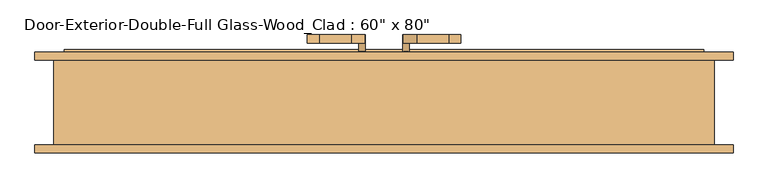
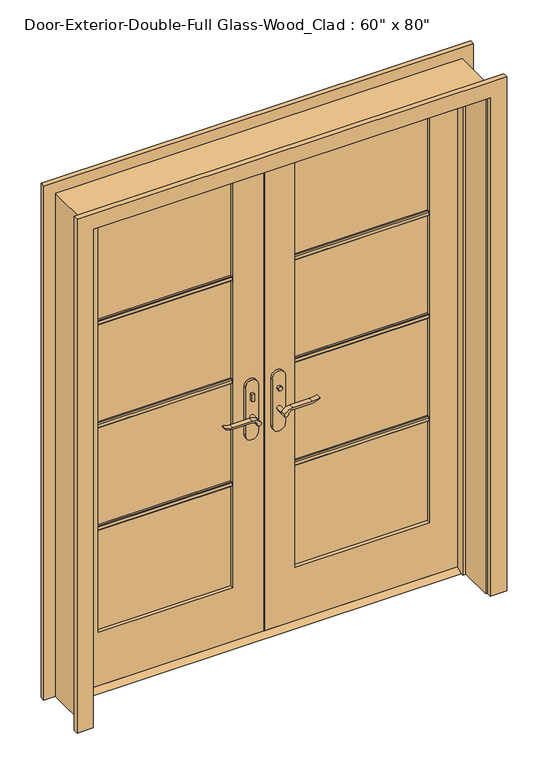
"""IFC4 building model written with IfcOpenShell, lengths in millimetres: door geometry."""

from ifc_helpers import new_model, si_unit, point, frame, frame_2d, origin, place, context, project, spatial, polyline, circle_curve, trimmed, segment, composite_curve, outline, extrude, faceted_brep, source, transform, mapped, element, save


def door_b03bd389(model_context):
    return source(origin(), model_context, "Body", "SolidModel", [
        extrude(outline(polyline([(63.5, 12.7), (98.425, 12.7), (123.825, 0.0), (38.1, 0.0), (63.5, 12.7)])), frame((-762.0, 0.0, 0.0), z_axis=(1.0, 0.0, 0.0), x_axis=(0.0, 1.0, 0.0)), (0.0, 0.0, 1.0), 1524.0),
        extrude(outline(polyline([(-47.4019111, 43.5), (-57.4019111, 43.5), (-57.4019111, 53.5), (-47.4019111, 53.5), (-47.4019111, 43.5)])), frame((0.0, 0.0, 981.9), z_axis=(0.0, 0.0, 1.0), x_axis=(1.0, 0.0, 0.0)), (0.0, 0.0, 1.0), 30.0),
        extrude(outline(composite_curve([segment(trimmed(circle_curve(frame_2d((996.9, -52.4019111)), 8.0), [point((996.9, -60.4019111))], [point((996.9, -44.4019111))], False, "CARTESIAN"), True, "CONTINUOUS"), segment(trimmed(circle_curve(frame_2d((996.9, -52.4019111)), 8.0), [point((996.9, -44.4019111))], [point((996.9, -60.4019111))], False, "CARTESIAN"), True, "CONTINUOUS")], self_intersect=False)), frame((0.0, 108.425, 0.0), z_axis=(0.0, 1.0, 0.0), x_axis=(0.0, 0.0, 1.0)), (0.0, 0.0, 1.0), 10.0),
        extrude(outline(composite_curve([segment(trimmed(circle_curve(frame_2d((897.1555521, -76.0694241)), 37.2832219), [point((919.0523287, -45.8937749))], [point((934.4, -77.7693445))], False, "CARTESIAN"), True, "CONTINUOUS"), segment(polyline([(934.4, -77.7693445), (934.4, -154.045502)]), True, "CONTINUOUS"), segment(trimmed(circle_curve(frame_2d((1017.6850638, -153.9791202)), 83.2850902), [point((934.4, -154.045502))], [point((939.4, -182.4019111))], True, "CARTESIAN"), True, "CONTINUOUS"), segment(polyline([(939.4, -182.4019111), (936.6135558, -182.4019111)]), True, "CONTINUOUS"), segment(trimmed(circle_curve(frame_2d((986.6709207, -150.4622499)), 59.3791355), [point((936.6135558, -182.4019111))], [point((927.4, -154.045502))], False, "CARTESIAN"), True, "CONTINUOUS"), segment(polyline([(927.4, -154.045502), (927.4, -77.7881013)]), True, "CONTINUOUS"), segment(trimmed(circle_curve(frame_2d((909.2738613, -77.7881013)), 18.1261387), [point((927.4, -77.7881013))], [point((914.4, -60.4019111))], True, "CARTESIAN"), True, "CONTINUOUS"), segment(trimmed(circle_curve(frame_2d((914.4, -52.4019111)), 8.0), [point((914.4, -60.4019111))], [point((919.0523287, -45.8937749))], False, "CARTESIAN"), True, "CONTINUOUS")], self_intersect=False)), frame((0.0, 3.5, 0.0), z_axis=(0.0, 1.0, 0.0), x_axis=(0.0, 0.0, 1.0)), (0.0, 0.0, 1.0), 20.0),
        extrude(outline(composite_curve([segment(trimmed(circle_curve(frame_2d((914.4, -52.4019111)), 8.0), [point((914.3999903, -60.4019111))], [point((919.0523287, -45.8937749))], False, "CARTESIAN"), True, "CONTINUOUS"), segment(trimmed(circle_curve(frame_2d((897.1555521, -76.0694241)), 37.2832219), [point((919.0523287, -45.8937749))], [point((934.4, -77.7693445))], False, "CARTESIAN"), True, "CONTINUOUS"), segment(polyline([(934.4, -77.7693445), (934.4, -154.045502)]), True, "CONTINUOUS"), segment(trimmed(circle_curve(frame_2d((1017.6850638, -153.9791202)), 83.2850902), [point((934.4, -154.045502))], [point((939.4, -182.4019111))], True, "CARTESIAN"), True, "CONTINUOUS"), segment(polyline([(939.4, -182.4019111), (936.6135558, -182.4019111)]), True, "CONTINUOUS"), segment(trimmed(circle_curve(frame_2d((986.6709207, -150.4622499)), 59.3791355), [point((936.6135558, -182.4019111))], [point((927.4, -154.045502))], False, "CARTESIAN"), True, "CONTINUOUS"), segment(polyline([(927.4, -154.045502), (927.4, -77.788099)]), True, "CONTINUOUS"), segment(trimmed(circle_curve(frame_2d((909.2738682, -77.788099)), 18.1261318), [point((927.4, -77.788099))], [point((914.3999903, -60.4019111))], True, "CARTESIAN"), True, "CONTINUOUS")], self_intersect=False)), frame((0.0, 138.425, 0.0), z_axis=(0.0, 1.0, 0.0), x_axis=(0.0, 0.0, 1.0)), (0.0, 0.0, 1.0), 20.0),
        extrude(outline(composite_curve([segment(trimmed(circle_curve(frame_2d((914.4, -52.4019111)), 8.0), [point((914.4, -60.4019111))], [point((914.4, -44.4019111))], False, "CARTESIAN"), True, "CONTINUOUS"), segment(trimmed(circle_curve(frame_2d((914.4, -52.4019111)), 8.0), [point((914.4, -44.4019111))], [point((914.4, -60.4019111))], False, "CARTESIAN"), True, "CONTINUOUS")], self_intersect=False)), frame((0.0, 23.5, 0.0), z_axis=(0.0, 1.0, 0.0), x_axis=(0.0, 0.0, 1.0)), (0.0, 0.0, 1.0), 30.0),
        extrude(outline(composite_curve([segment(trimmed(circle_curve(frame_2d((914.4, -52.4019111)), 8.0), [point((914.4, -60.4019111))], [point((914.4, -44.4019111))], False, "CARTESIAN"), True, "CONTINUOUS"), segment(trimmed(circle_curve(frame_2d((914.4, -52.4019111)), 8.0), [point((914.4, -44.4019111))], [point((914.4, -60.4019111))], False, "CARTESIAN"), True, "CONTINUOUS")], self_intersect=False)), frame((0.0, 108.425, 0.0), z_axis=(0.0, 1.0, 0.0), x_axis=(0.0, 0.0, 1.0)), (0.0, 0.0, 1.0), 30.0),
        extrude(outline(composite_curve([segment(polyline([(844.4, -27.4019111), (1039.4, -27.4019111)]), True, "CONTINUOUS"), segment(trimmed(circle_curve(frame_2d((1039.4, -52.4019111)), 25.0), [point((1039.4, -27.4019111))], [point((1039.4, -77.4019111))], False, "CARTESIAN"), True, "CONTINUOUS"), segment(polyline([(1039.4, -77.4019111), (844.4, -77.4019111)]), True, "CONTINUOUS"), segment(trimmed(circle_curve(frame_2d((844.4, -52.4019111)), 25.0), [point((844.4, -77.4019111))], [point((844.4, -27.4019111))], False, "CARTESIAN"), True, "CONTINUOUS")], self_intersect=False)), frame((0.0, 53.5, 0.0), z_axis=(0.0, 1.0, 0.0), x_axis=(0.0, 0.0, 1.0)), (0.0, 0.0, 1.0), 10.0),
        extrude(outline(composite_curve([segment(polyline([(844.4, -27.4019111), (1039.4, -27.4019111)]), True, "CONTINUOUS"), segment(trimmed(circle_curve(frame_2d((1039.4, -52.4019111)), 25.0), [point((1039.4, -27.4019111))], [point((1039.4, -77.4019111))], False, "CARTESIAN"), True, "CONTINUOUS"), segment(polyline([(1039.4, -77.4019111), (844.4, -77.4019111)]), True, "CONTINUOUS"), segment(trimmed(circle_curve(frame_2d((844.4, -52.4019111)), 25.0), [point((844.4, -77.4019111))], [point((844.4, -27.4019111))], False, "CARTESIAN"), True, "CONTINUOUS")], self_intersect=False)), frame((0.0, 98.425, 0.0), z_axis=(0.0, 1.0, 0.0), x_axis=(0.0, 0.0, 1.0)), (0.0, 0.0, 1.0), 10.0),
        extrude(outline(polyline([(47.3875, 118.425), (57.3875, 118.425), (57.3875, 108.425), (47.3875, 108.425), (47.3875, 118.425)])), frame((0.0, 0.0, 981.9), z_axis=(0.0, 0.0, 1.0), x_axis=(1.0, 0.0, 0.0)), (0.0, 0.0, 1.0), 30.0),
        extrude(outline(composite_curve([segment(trimmed(circle_curve(frame_2d((996.9, 52.3875)), 8.0), [point((996.9, 60.3875))], [point((996.9, 44.3875))], False, "CARTESIAN"), True, "CONTINUOUS"), segment(trimmed(circle_curve(frame_2d((996.9, 52.3875)), 8.0), [point((996.9, 44.3875))], [point((996.9, 60.3875))], False, "CARTESIAN"), True, "CONTINUOUS")], self_intersect=False)), frame((0.0, 43.5, 0.0), z_axis=(0.0, 1.0, 0.0), x_axis=(0.0, 0.0, 1.0)), (0.0, 0.0, 1.0), 10.0),
        extrude(outline(composite_curve([segment(trimmed(circle_curve(frame_2d((914.4, 52.3875)), 8.0), [point((919.0523287, 45.8793637))], [point((914.4, 60.3875))], False, "CARTESIAN"), True, "CONTINUOUS"), segment(trimmed(circle_curve(frame_2d((909.2738613, 77.7736901)), 18.1261387), [point((914.4, 60.3875))], [point((927.4, 77.7736901))], True, "CARTESIAN"), True, "CONTINUOUS"), segment(polyline([(927.4, 77.7736901), (927.4, 154.0310909)]), True, "CONTINUOUS"), segment(trimmed(circle_curve(frame_2d((986.6709207, 150.4478388)), 59.3791355), [point((927.4, 154.0310909))], [point((936.6135558, 182.3875))], False, "CARTESIAN"), True, "CONTINUOUS"), segment(polyline([(936.6135558, 182.3875), (939.4, 182.3875)]), True, "CONTINUOUS"), segment(trimmed(circle_curve(frame_2d((1017.6850638, 153.9647091)), 83.2850902), [point((939.4, 182.3875))], [point((934.4, 154.0310909))], True, "CARTESIAN"), True, "CONTINUOUS"), segment(polyline([(934.4, 154.0310909), (934.4, 77.7549333)]), True, "CONTINUOUS"), segment(trimmed(circle_curve(frame_2d((897.1555521, 76.0550129)), 37.2832219), [point((934.4, 77.7549333))], [point((919.0523287, 45.8793637))], False, "CARTESIAN"), True, "CONTINUOUS")], self_intersect=False)), frame((0.0, 138.425, 0.0), z_axis=(0.0, 1.0, 0.0), x_axis=(0.0, 0.0, 1.0)), (0.0, 0.0, 1.0), 20.0),
        extrude(outline(composite_curve([segment(trimmed(circle_curve(frame_2d((909.2738682, 77.7736878)), 18.1261318), [point((914.3999903, 60.3875))], [point((927.4, 77.7736878))], True, "CARTESIAN"), True, "CONTINUOUS"), segment(polyline([(927.4, 77.7736878), (927.4, 154.0310909)]), True, "CONTINUOUS"), segment(trimmed(circle_curve(frame_2d((986.6709207, 150.4478388)), 59.3791355), [point((927.4, 154.0310909))], [point((936.6135558, 182.3875))], False, "CARTESIAN"), True, "CONTINUOUS"), segment(polyline([(936.6135558, 182.3875), (939.4, 182.3875)]), True, "CONTINUOUS"), segment(trimmed(circle_curve(frame_2d((1017.6850638, 153.9647091)), 83.2850902), [point((939.4, 182.3875))], [point((934.4, 154.0310909))], True, "CARTESIAN"), True, "CONTINUOUS"), segment(polyline([(934.4, 154.0310909), (934.4, 77.7549333)]), True, "CONTINUOUS"), segment(trimmed(circle_curve(frame_2d((897.1555521, 76.0550129)), 37.2832219), [point((934.4, 77.7549333))], [point((919.0523287, 45.8793637))], False, "CARTESIAN"), True, "CONTINUOUS"), segment(trimmed(circle_curve(frame_2d((914.4, 52.3875)), 8.0), [point((919.0523287, 45.8793637))], [point((914.3999903, 60.3875))], False, "CARTESIAN"), True, "CONTINUOUS")], self_intersect=False)), frame((0.0, 3.5, 0.0), z_axis=(0.0, 1.0, 0.0), x_axis=(0.0, 0.0, 1.0)), (0.0, 0.0, 1.0), 20.0),
        extrude(outline(composite_curve([segment(trimmed(circle_curve(frame_2d((914.4, 52.3875)), 8.0), [point((914.4, 60.3875))], [point((914.4, 44.3875))], False, "CARTESIAN"), True, "CONTINUOUS"), segment(trimmed(circle_curve(frame_2d((914.4, 52.3875)), 8.0), [point((914.4, 44.3875))], [point((914.4, 60.3875))], False, "CARTESIAN"), True, "CONTINUOUS")], self_intersect=False)), frame((0.0, 108.425, 0.0), z_axis=(0.0, 1.0, 0.0), x_axis=(0.0, 0.0, 1.0)), (0.0, 0.0, 1.0), 30.0),
        extrude(outline(composite_curve([segment(trimmed(circle_curve(frame_2d((914.4, 52.3875)), 8.0), [point((914.4, 60.3875))], [point((914.4, 44.3875))], False, "CARTESIAN"), True, "CONTINUOUS"), segment(trimmed(circle_curve(frame_2d((914.4, 52.3875)), 8.0), [point((914.4, 44.3875))], [point((914.4, 60.3875))], False, "CARTESIAN"), True, "CONTINUOUS")], self_intersect=False)), frame((0.0, 23.5, 0.0), z_axis=(0.0, 1.0, 0.0), x_axis=(0.0, 0.0, 1.0)), (0.0, 0.0, 1.0), 30.0),
        extrude(outline(composite_curve([segment(trimmed(circle_curve(frame_2d((844.4, 52.3875)), 25.0), [point((844.4, 27.3875))], [point((844.4, 77.3875))], False, "CARTESIAN"), True, "CONTINUOUS"), segment(polyline([(844.4, 77.3875), (1039.4, 77.3875)]), True, "CONTINUOUS"), segment(trimmed(circle_curve(frame_2d((1039.4, 52.3875)), 25.0), [point((1039.4, 77.3875))], [point((1039.4, 27.3875))], False, "CARTESIAN"), True, "CONTINUOUS"), segment(polyline([(1039.4, 27.3875), (844.4, 27.3875)]), True, "CONTINUOUS")], self_intersect=False)), frame((0.0, 98.425, 0.0), z_axis=(0.0, 1.0, 0.0), x_axis=(0.0, 0.0, 1.0)), (0.0, 0.0, 1.0), 10.0),
        extrude(outline(composite_curve([segment(trimmed(circle_curve(frame_2d((844.4, 52.3875)), 25.0), [point((844.4, 27.3875))], [point((844.4, 77.3875))], False, "CARTESIAN"), True, "CONTINUOUS"), segment(polyline([(844.4, 77.3875), (1039.4, 77.3875)]), True, "CONTINUOUS"), segment(trimmed(circle_curve(frame_2d((1039.4, 52.3875)), 25.0), [point((1039.4, 77.3875))], [point((1039.4, 27.3875))], False, "CARTESIAN"), True, "CONTINUOUS"), segment(polyline([(1039.4, 27.3875), (844.4, 27.3875)]), True, "CONTINUOUS")], self_intersect=False)), frame((0.0, 53.5, 0.0), z_axis=(0.0, 1.0, 0.0), x_axis=(0.0, 0.0, 1.0)), (0.0, 0.0, 1.0), 10.0),
        extrude(outline(polyline([(77.47, 1502.171875), (77.47, 1483.121875), (71.12, 1483.121875), (67.945, 1486.296875), (67.945, 1498.996875), (71.12, 1502.171875), (77.47, 1502.171875)])), frame((120.65, 0.0, 0.0), z_axis=(1.0, 0.0, 0.0), x_axis=(0.0, 1.0, 0.0)), (0.0, 0.0, 1.0), 520.7),
        extrude(outline(polyline([(77.47, 1081.88125), (77.47, 1062.83125), (71.12, 1062.83125), (67.945, 1066.00625), (67.945, 1078.70625), (71.12, 1081.88125), (77.47, 1081.88125)])), frame((120.65, 0.0, 0.0), z_axis=(1.0, 0.0, 0.0), x_axis=(0.0, 1.0, 0.0)), (0.0, 0.0, 1.0), 520.7),
        extrude(outline(polyline([(77.47, 661.590625), (77.47, 642.540625), (71.12, 642.540625), (67.945, 645.715625), (67.945, 658.415625), (71.12, 661.590625), (77.47, 661.590625)])), frame((120.65, 0.0, 0.0), z_axis=(1.0, 0.0, 0.0), x_axis=(0.0, 1.0, 0.0)), (0.0, 0.0, 1.0), 520.7),
        extrude(outline(polyline([(84.455, 1502.171875), (90.805, 1502.171875), (93.98, 1498.996875), (93.98, 1486.296875), (90.805, 1483.121875), (84.455, 1483.121875), (84.455, 1502.171875)])), frame((-641.35, 0.0, 0.0), z_axis=(1.0, 0.0, 0.0), x_axis=(0.0, 1.0, 0.0)), (0.0, 0.0, 1.0), 520.7),
        extrude(outline(polyline([(84.455, 1081.88125), (90.805, 1081.88125), (93.98, 1078.70625), (93.98, 1066.00625), (90.805, 1062.83125), (84.455, 1062.83125), (84.455, 1081.88125)])), frame((-641.35, 0.0, 0.0), z_axis=(1.0, 0.0, 0.0), x_axis=(0.0, 1.0, 0.0)), (0.0, 0.0, 1.0), 520.7),
        extrude(outline(polyline([(84.455, 661.590625), (90.805, 661.590625), (93.98, 658.415625), (93.98, 645.715625), (90.805, 642.540625), (84.455, 642.540625), (84.455, 661.590625)])), frame((-641.35, 0.0, 0.0), z_axis=(1.0, 0.0, 0.0), x_axis=(0.0, 1.0, 0.0)), (0.0, 0.0, 1.0), 520.7),
        extrude(outline(polyline([(84.455, 1502.171875), (90.805, 1502.171875), (93.98, 1498.996875), (93.98, 1486.296875), (90.805, 1483.121875), (84.455, 1483.121875), (84.455, 1502.171875)])), frame((120.65, 0.0, 0.0), z_axis=(1.0, 0.0, 0.0), x_axis=(0.0, 1.0, 0.0)), (0.0, 0.0, 1.0), 520.7),
        extrude(outline(polyline([(84.455, 1081.88125), (90.805, 1081.88125), (93.98, 1078.70625), (93.98, 1066.00625), (90.805, 1062.83125), (84.455, 1062.83125), (84.455, 1081.88125)])), frame((120.65, 0.0, 0.0), z_axis=(1.0, 0.0, 0.0), x_axis=(0.0, 1.0, 0.0)), (0.0, 0.0, 1.0), 520.7),
        extrude(outline(polyline([(84.455, 661.590625), (90.805, 661.590625), (93.98, 658.415625), (93.98, 645.715625), (90.805, 642.540625), (84.455, 642.540625), (84.455, 661.590625)])), frame((120.65, 0.0, 0.0), z_axis=(1.0, 0.0, 0.0), x_axis=(0.0, 1.0, 0.0)), (0.0, 0.0, 1.0), 520.7),
        extrude(outline(polyline([(77.47, 1502.171875), (77.47, 1483.121875), (71.12, 1483.121875), (67.945, 1486.296875), (67.945, 1498.996875), (71.12, 1502.171875), (77.47, 1502.171875)])), frame((-641.35, 0.0, 0.0), z_axis=(1.0, 0.0, 0.0), x_axis=(0.0, 1.0, 0.0)), (0.0, 0.0, 1.0), 520.7),
        extrude(outline(polyline([(77.47, 1081.88125), (77.47, 1062.83125), (71.12, 1062.83125), (67.945, 1066.00625), (67.945, 1078.70625), (71.12, 1081.88125), (77.47, 1081.88125)])), frame((-641.35, 0.0, 0.0), z_axis=(1.0, 0.0, 0.0), x_axis=(0.0, 1.0, 0.0)), (0.0, 0.0, 1.0), 520.7),
        extrude(outline(polyline([(77.47, 661.590625), (77.47, 642.540625), (71.12, 642.540625), (67.945, 645.715625), (67.945, 658.415625), (71.12, 661.590625), (77.47, 661.590625)])), frame((-641.35, 0.0, 0.0), z_axis=(1.0, 0.0, 0.0), x_axis=(0.0, 1.0, 0.0)), (0.0, 0.0, 1.0), 520.7),
        extrude(outline(polyline([(0.0, 768.35), (0.0, 831.85), (2101.85, 831.85), (2101.85, -831.85), (0.0, -831.85), (0.0, -768.35), (2038.35, -768.35), (2038.35, 768.35), (0.0, 768.35)])), frame((0.0, 98.425, 0.0), z_axis=(0.0, 1.0, 0.0), x_axis=(0.0, 0.0, 1.0)), (0.0, 0.0, 1.0), 19.05),
        extrude(outline(polyline([(0.0, 768.35), (0.0, 831.85), (2101.85, 831.85), (2101.85, -831.85), (0.0, -831.85), (0.0, -768.35), (2038.35, -768.35), (2038.35, 768.35), (0.0, 768.35)])), frame((0.0, -123.825, 0.0), z_axis=(0.0, 1.0, 0.0), x_axis=(0.0, 0.0, 1.0)), (0.0, 0.0, 1.0), 19.05),
        extrude(outline(polyline([(12.7, 762.0), (2032.0, 762.0), (2032.0, 1.5875), (12.7, 1.5875), (12.7, 762.0)]), holes=[polyline([(1912.9375, 120.65), (1912.9375, 641.35), (231.775, 641.35), (231.775, 120.65), (1912.9375, 120.65)])]), frame((0.0, 63.5, 0.0), z_axis=(0.0, 1.0, 0.0), x_axis=(0.0, 0.0, 1.0)), (0.0, 0.0, 1.0), 34.925),
        extrude(outline(polyline([(2032.0, -762.0), (12.7, -762.0), (12.7, -1.6019111), (2032.0, -1.6019111), (2032.0, -762.0)]), holes=[polyline([(231.775, -641.35), (1912.9375, -641.35), (1912.9375, -120.65), (231.775, -120.65), (231.775, -641.35)])]), frame((0.0, 63.5, 0.0), z_axis=(0.0, 1.0, 0.0), x_axis=(0.0, 0.0, 1.0)), (0.0, 0.0, 1.0), 34.925),
        faceted_brep([(787.4, 98.425, 0.0), (787.4, -104.775, 0.0), (762.0, -104.775, 0.0), (762.0, 28.575, 0.0), (749.3, 28.575, 0.0), (749.3, 63.5, 0.0), (762.0, 63.5, 0.0), (762.0, 98.425, 0.0), (787.4, 98.425, 2057.4), (787.4, -104.775, 2057.4), (-787.4, -104.775, 2057.4), (-787.4, -104.775, 0.0), (-762.0, -104.775, 0.0), (-762.0, -104.775, 2032.0), (762.0, -104.775, 2032.0), (762.0, 28.575, 2032.0), (-762.0, 28.575, 2032.0), (-762.0, 28.575, 0.0), (-749.3, 28.575, 0.0), (-749.3, 28.575, 2019.3), (749.3, 28.575, 2019.3), (749.3, 63.5, 2019.3), (1.5875, 63.5, 2019.3), (-1.6019111, 63.5, 2019.3), (-749.3, 63.5, 2019.3), (-749.3, 63.5, 0.0), (-762.0, 63.5, 0.0), (-762.0, 63.5, 2032.0), (-1.6019111, 63.5, 2032.0), (1.5875, 63.5, 2032.0), (762.0, 63.5, 2032.0), (762.0, 98.425, 2032.0), (1.5875, 98.425, 2032.0), (-1.6019111, 98.425, 2032.0), (-762.0, 98.425, 2032.0), (-762.0, 98.425, 0.0), (-787.4, 98.425, 0.0), (-787.4, 98.425, 2057.4)], [[[0, 1, 2, 3, 4, 5, 6, 7]], [[1, 0, 8, 9]], [[2, 1, 9, 10, 11, 12, 13, 14]], [[3, 2, 14, 15]], [[4, 3, 15, 16, 17, 18, 19, 20]], [[5, 4, 20, 21]], [[6, 5, 21, 22, 23, 24, 25, 26, 27, 28, 29, 30]], [[7, 6, 30, 31]], [[0, 7, 31, 32, 33, 34, 35, 36, 37, 8]], [[9, 8, 37, 10]], [[14, 13, 16, 15]], [[20, 19, 24, 23, 22, 21]], [[31, 30, 29, 28, 27, 34, 33, 32]], [[12, 11, 36, 35, 26, 25, 18, 17]], [[11, 10, 37, 36]], [[13, 12, 17, 16]], [[19, 18, 25, 24]], [[27, 26, 35, 34]]]),
        extrude(outline(polyline([(641.35, 77.47), (120.65, 77.47), (120.65, 84.455), (641.35, 84.455), (641.35, 77.47)])), frame((0.0, 0.0, 231.775), z_axis=(0.0, 0.0, 1.0), x_axis=(1.0, 0.0, 0.0)), (0.0, 0.0, 1.0), 1681.1625),
        extrude(outline(polyline([(-120.65, 77.47), (-641.35, 77.47), (-641.35, 84.455), (-120.65, 84.455), (-120.65, 77.47)])), frame((0.0, 0.0, 231.775), z_axis=(0.0, 0.0, 1.0), x_axis=(1.0, 0.0, 0.0)), (0.0, 0.0, 1.0), 1681.1625),
    ])


if __name__ == "__main__":
    model = new_model("IFC4")
    model_context = context("Model", 3, world=origin())
    ifc_project = project(units=[si_unit("LENGTHUNIT", "METRE", prefix="MILLI")], contexts=[model_context])
    site = spatial("IfcSite", under=ifc_project)
    building = spatial("IfcBuilding", under=site)
    placement = place(None, origin())
    door_shape = door_b03bd389(model_context)
    element("IfcDoor", 1, ObjectType="Door-Exterior-Double-Full Glass-Wood_Clad : 60\" x 80\"", at=placement, inside=building, context=model_context, shape_type="MappedRepresentation", body=[
        mapped(door_shape, transform((0.0, 0.0, 0.0), x_axis=(1.0, 0.0, 0.0), y_axis=(0.0, 1.0, 0.0), z_axis=(0.0, 0.0, 1.0))),
    ])
    save(model, "model.ifc")

# Revit data of these elements
# Type "Door-Exterior-Double-Full Glass-Wood_Clad : 60\" x 80\""
#   Type Mark = "8"
#   Assembly Code = "B2030100"
#   Analytic Construction = "French door, wood frame with double glass"
#   Top Rail = 0' - 4 11/16"
#   Threshold Offset [instance default] = 0' - 0 1/2"
#   Thickness = 0' - 1 3/8"
#   Thermal Resistance (R) = 1.9158 (h·ft²·°F)/BTU
#   Swing Angle [instance default] = 90.00°
#   Stiles = 0' - 4 3/4"
#   Rough Width = 5' - 2"
#   Rough Height = 6' - 9"
#   Panel Width = 2' - 6"
#   Door Offset [instance default] = 0' - 0"
#   Height = 6' - 8"
#   Width = 5' - 0"
#   Heat Transfer Coefficient (U) = 0.5220 BTU/(h·ft²·°F)
#   Bottom Rail = 0' - 9 1/8"
#   Exterior Trim [instance default] = yes
#   Threshold [instance default] = yes
#   Show Grill [instance default] = yes
#   Function = 1
#   Trim Material = Cherry
#   Threshold Material = Cherry
#   Panel Material = Cherry
#   Glazing = Glass
#   Frame Material = Cherry
#   Door Handle Material = Aluminum
#   Visual Light Transmittance = 0
#   Solar Heat Gain Coefficient = 0
#   Wall Closure = (empty or 0)
#   Construction Type = (empty or 0)
# Element 1 (IfcDoor, "Door-Exterior-Double-Full Glass-Wood_Clad : 60\" x 80\"")
#   Materials on its faces: "Cherry", "Aluminum", "Glass"
# Materials
#   "Cherry": class "Wood", colour RGB 226 177 128, transparency 0, Description = "Prunus Serotina", Cost = 0
#   "Glass": class "Glass", colour RGB 0 128 192, transparency 0.75, Description = "Soda Lime Glass", Cost = 0
#   "Aluminum": class "Metal", colour RGB 247 247 247, transparency 0, Description = "Aluminum 6061", Cost = 0
